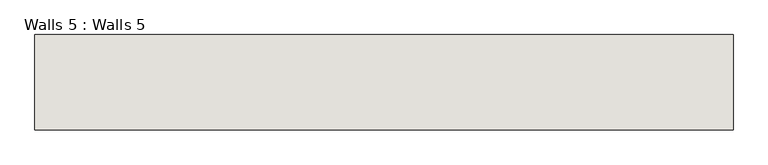
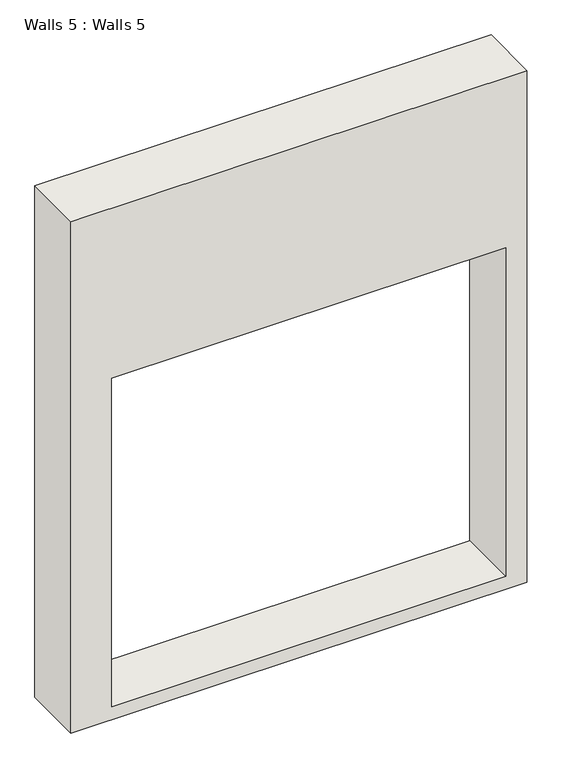
"""IFC4 building model written with IfcOpenShell, lengths in millimetres: wall geometry, Walls 5 : Walls 5."""

from ifc_helpers import new_model, si_unit, frame, origin, place, context, project, spatial, polyline, outline, extrude, source, transform, mapped, element, save


def walls_5_walls_5_ae1c99f5(model_context):
    return source(origin(), model_context, "Body", "SweptSolid", [
        extrude(outline(polyline([(0.0, -9880.3407032), (0.0, -7646.7407032), (2648.0, -7646.7407032), (2648.0, -9880.3407032), (0.0, -9880.3407032)]), holes=[polyline([(65.8898568, -9680.3407032), (1767.6898568, -9680.3407032), (1767.6898568, -7749.9407032), (65.8898568, -7749.9407032), (65.8898568, -9680.3407032)])]), frame((0.0, 3656.1956099, 0.0), z_axis=(0.0, 1.0, 0.0), x_axis=(0.0, 0.0, 1.0)), (0.0, 0.0, 1.0), 304.8),
    ])


if __name__ == "__main__":
    model = new_model("IFC4")
    model_context = context("Model", 3, world=origin())
    ifc_project = project(units=[si_unit("LENGTHUNIT", "METRE", prefix="MILLI")], contexts=[model_context])
    site = spatial("IfcSite", under=ifc_project)
    building = spatial("IfcBuilding", under=site)
    placement = place(None, origin())
    walls_5_walls_5_shape = walls_5_walls_5_ae1c99f5(model_context)
    element("IfcWall", 1, ObjectType="Walls 5 : Walls 5", at=placement, inside=building, context=model_context, shape_type="MappedRepresentation", body=[
        mapped(walls_5_walls_5_shape, transform((0.0, 0.0, 0.0), x_axis=(1.0, 0.0, 0.0), y_axis=(0.0, 1.0, 0.0), z_axis=(0.0, 0.0, 1.0))),
    ])
    save(model, "model.ifc")

# Revit data of these elements
# Element 1 (IfcWall, "Walls 5 : Walls 5")
#   Materials on its faces: "Default Wall"
# Materials
#   "Default Wall": colour RGB 80 80 80, transparency 0
